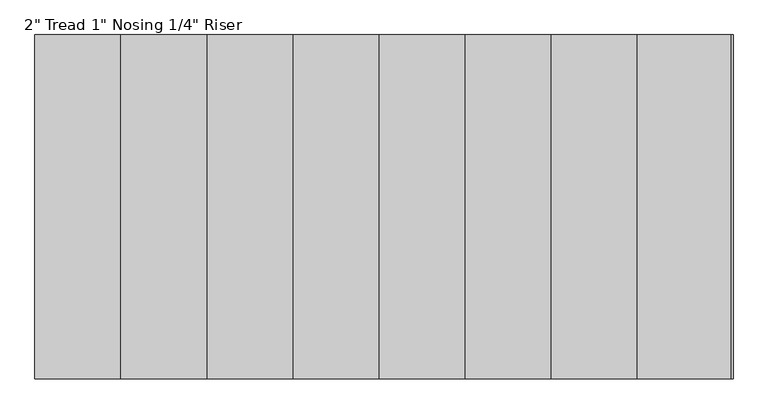
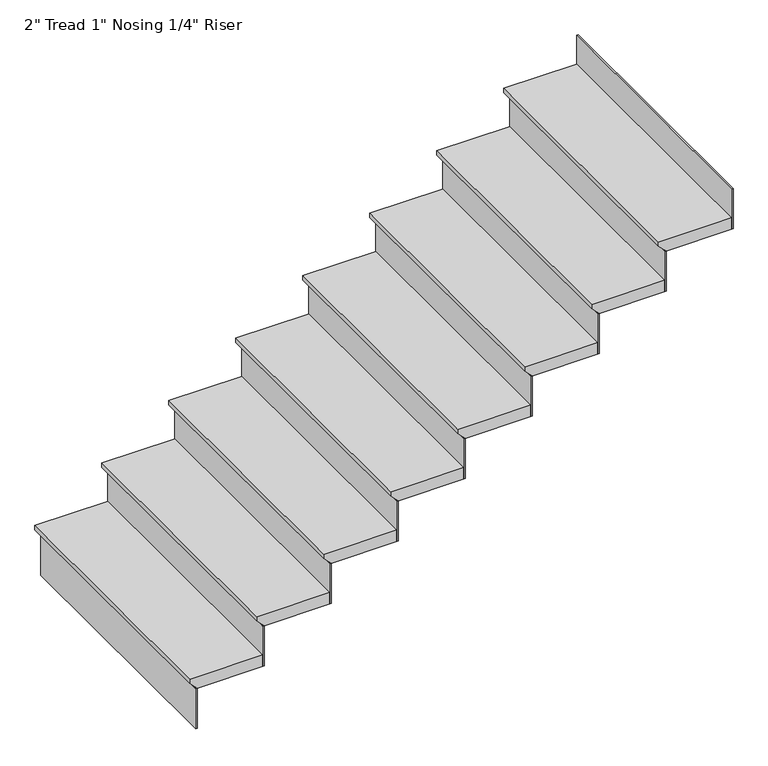
"""IFC4 building model written with IfcOpenShell, lengths in millimetres: stair flight geometry."""

from ifc_helpers import new_model, si_unit, frame, origin, place, context, project, spatial, polyline, outline, extrude, source, transform, mapped, element, save


def stair_flight_53bbb6a0(model_context):
    return source(origin(), model_context, "Body", "SweptSolid", [
        extrude(outline(polyline([(4978.4, -9891.2683044), (4978.4, -10196.0683044), (4959.35, -10196.0683044), (4933.95, -10170.6683044), (4927.6, -10170.6683044), (4927.6, -9891.2683044), (4978.4, -9891.2683044)])), frame((0.0, -2492.1891189, 0.0), z_axis=(0.0, 1.0, 0.0), x_axis=(0.0, 0.0, 1.0)), (0.0, 0.0, 1.0), 1117.6),
        extrude(outline(polyline([(-10164.3183044, -2492.1891189), (-10170.6683044, -2492.1891189), (-10170.6683044, -1374.5891189), (-10164.3183044, -1374.5891189), (-10164.3183044, -2492.1891189)])), frame((0.0, 0.0, 4749.8), z_axis=(0.0, 0.0, 1.0), x_axis=(1.0, 0.0, 0.0)), (0.0, 0.0, 1.0), 177.8),
        extrude(outline(polyline([(-9884.9183044, -2492.1891189), (-9891.2683044, -2492.1891189), (-9891.2683044, -1374.5891189), (-9884.9183044, -1374.5891189), (-9884.9183044, -2492.1891189)])), frame((0.0, 0.0, 4927.6), z_axis=(0.0, 0.0, 1.0), x_axis=(1.0, 0.0, 0.0)), (0.0, 0.0, 1.0), 177.8),
        extrude(outline(polyline([(5156.2, -9611.8683044), (5156.2, -9916.6683044), (5137.15, -9916.6683044), (5111.75, -9891.2683044), (5105.4, -9891.2683044), (5105.4, -9611.8683044), (5156.2, -9611.8683044)])), frame((0.0, -2492.1891189, 0.0), z_axis=(0.0, 1.0, 0.0), x_axis=(0.0, 0.0, 1.0)), (0.0, 0.0, 1.0), 1117.6),
        extrude(outline(polyline([(-9605.5183044, -2492.1891189), (-9611.8683044, -2492.1891189), (-9611.8683044, -1374.5891189), (-9605.5183044, -1374.5891189), (-9605.5183044, -2492.1891189)])), frame((0.0, 0.0, 5105.4), z_axis=(0.0, 0.0, 1.0), x_axis=(1.0, 0.0, 0.0)), (0.0, 0.0, 1.0), 177.8),
        extrude(outline(polyline([(5334.0, -9332.4683044), (5334.0, -9637.2683044), (5314.95, -9637.2683044), (5289.55, -9611.8683044), (5283.2, -9611.8683044), (5283.2, -9332.4683044), (5334.0, -9332.4683044)])), frame((0.0, -2492.1891189, 0.0), z_axis=(0.0, 1.0, 0.0), x_axis=(0.0, 0.0, 1.0)), (0.0, 0.0, 1.0), 1117.6),
        extrude(outline(polyline([(-9326.1183044, -2492.1891189), (-9332.4683044, -2492.1891189), (-9332.4683044, -1374.5891189), (-9326.1183044, -1374.5891189), (-9326.1183044, -2492.1891189)])), frame((0.0, 0.0, 5283.2), z_axis=(0.0, 0.0, 1.0), x_axis=(1.0, 0.0, 0.0)), (0.0, 0.0, 1.0), 177.8),
        extrude(outline(polyline([(5511.8, -9053.0683044), (5511.8, -9357.8683044), (5492.75, -9357.8683044), (5467.35, -9332.4683044), (5461.0, -9332.4683044), (5461.0, -9053.0683044), (5511.8, -9053.0683044)])), frame((0.0, -2492.1891189, 0.0), z_axis=(0.0, 1.0, 0.0), x_axis=(0.0, 0.0, 1.0)), (0.0, 0.0, 1.0), 1117.6),
        extrude(outline(polyline([(-9046.7183044, -2492.1891189), (-9053.0683044, -2492.1891189), (-9053.0683044, -1374.5891189), (-9046.7183044, -1374.5891189), (-9046.7183044, -2492.1891189)])), frame((0.0, 0.0, 5461.0), z_axis=(0.0, 0.0, 1.0), x_axis=(1.0, 0.0, 0.0)), (0.0, 0.0, 1.0), 177.8),
        extrude(outline(polyline([(5689.6, -8773.6683044), (5689.6, -9078.4683044), (5670.55, -9078.4683044), (5645.15, -9053.0683044), (5638.8, -9053.0683044), (5638.8, -8773.6683044), (5689.6, -8773.6683044)])), frame((0.0, -2492.1891189, 0.0), z_axis=(0.0, 1.0, 0.0), x_axis=(0.0, 0.0, 1.0)), (0.0, 0.0, 1.0), 1117.6),
        extrude(outline(polyline([(-8767.3183044, -2492.1891189), (-8773.6683044, -2492.1891189), (-8773.6683044, -1374.5891189), (-8767.3183044, -1374.5891189), (-8767.3183044, -2492.1891189)])), frame((0.0, 0.0, 5638.8), z_axis=(0.0, 0.0, 1.0), x_axis=(1.0, 0.0, 0.0)), (0.0, 0.0, 1.0), 177.8),
        extrude(outline(polyline([(5867.4, -8494.2683044), (5867.4, -8799.0683044), (5848.35, -8799.0683044), (5822.95, -8773.6683044), (5816.6, -8773.6683044), (5816.6, -8494.2683044), (5867.4, -8494.2683044)])), frame((0.0, -2492.1891189, 0.0), z_axis=(0.0, 1.0, 0.0), x_axis=(0.0, 0.0, 1.0)), (0.0, 0.0, 1.0), 1117.6),
        extrude(outline(polyline([(-8487.9183044, -2492.1891189), (-8494.2683044, -2492.1891189), (-8494.2683044, -1374.5891189), (-8487.9183044, -1374.5891189), (-8487.9183044, -2492.1891189)])), frame((0.0, 0.0, 5816.6), z_axis=(0.0, 0.0, 1.0), x_axis=(1.0, 0.0, 0.0)), (0.0, 0.0, 1.0), 177.8),
        extrude(outline(polyline([(6045.2, -8214.8683044), (6045.2, -8519.6683044), (6026.15, -8519.6683044), (6000.75, -8494.2683044), (5994.4, -8494.2683044), (5994.4, -8214.8683044), (6045.2, -8214.8683044)])), frame((0.0, -2492.1891189, 0.0), z_axis=(0.0, 1.0, 0.0), x_axis=(0.0, 0.0, 1.0)), (0.0, 0.0, 1.0), 1117.6),
        extrude(outline(polyline([(-8208.5183044, -2492.1891189), (-8214.8683044, -2492.1891189), (-8214.8683044, -1374.5891189), (-8208.5183044, -1374.5891189), (-8208.5183044, -2492.1891189)])), frame((0.0, 0.0, 5994.4), z_axis=(0.0, 0.0, 1.0), x_axis=(1.0, 0.0, 0.0)), (0.0, 0.0, 1.0), 177.8),
        extrude(outline(polyline([(-7929.1183044, -2492.1891189), (-7935.4683044, -2492.1891189), (-7935.4683044, -1374.5891189), (-7929.1183044, -1374.5891189), (-7929.1183044, -2492.1891189)])), frame((0.0, 0.0, 6172.2), z_axis=(0.0, 0.0, 1.0), x_axis=(1.0, 0.0, 0.0)), (0.0, 0.0, 1.0), 177.8),
        extrude(outline(polyline([(6223.0, -7935.4683044), (6223.0, -8240.2683044), (6203.95, -8240.2683044), (6178.55, -8214.8683044), (6172.2, -8214.8683044), (6172.2, -7935.4683044), (6223.0, -7935.4683044)])), frame((0.0, -2492.1891189, 0.0), z_axis=(0.0, 1.0, 0.0), x_axis=(0.0, 0.0, 1.0)), (0.0, 0.0, 1.0), 1117.6),
    ])


if __name__ == "__main__":
    model = new_model("IFC4")
    model_context = context("Model", 3, world=origin())
    ifc_project = project(units=[si_unit("LENGTHUNIT", "METRE", prefix="MILLI")], contexts=[model_context])
    site = spatial("IfcSite", under=ifc_project)
    building = spatial("IfcBuilding", under=site)
    placement = place(None, origin())
    stair_flight_shape = stair_flight_53bbb6a0(model_context)
    element("IfcStairFlight", 1, ObjectType="2\" Tread 1\" Nosing 1/4\" Riser", at=placement, inside=building, context=model_context, shape_type="MappedRepresentation", body=[
        mapped(stair_flight_shape, transform((0.0, 0.0, 0.0), x_axis=(1.0, 0.0, 0.0), y_axis=(0.0, 1.0, 0.0), z_axis=(0.0, 0.0, 1.0))),
    ])
    save(model, "model.ifc")
